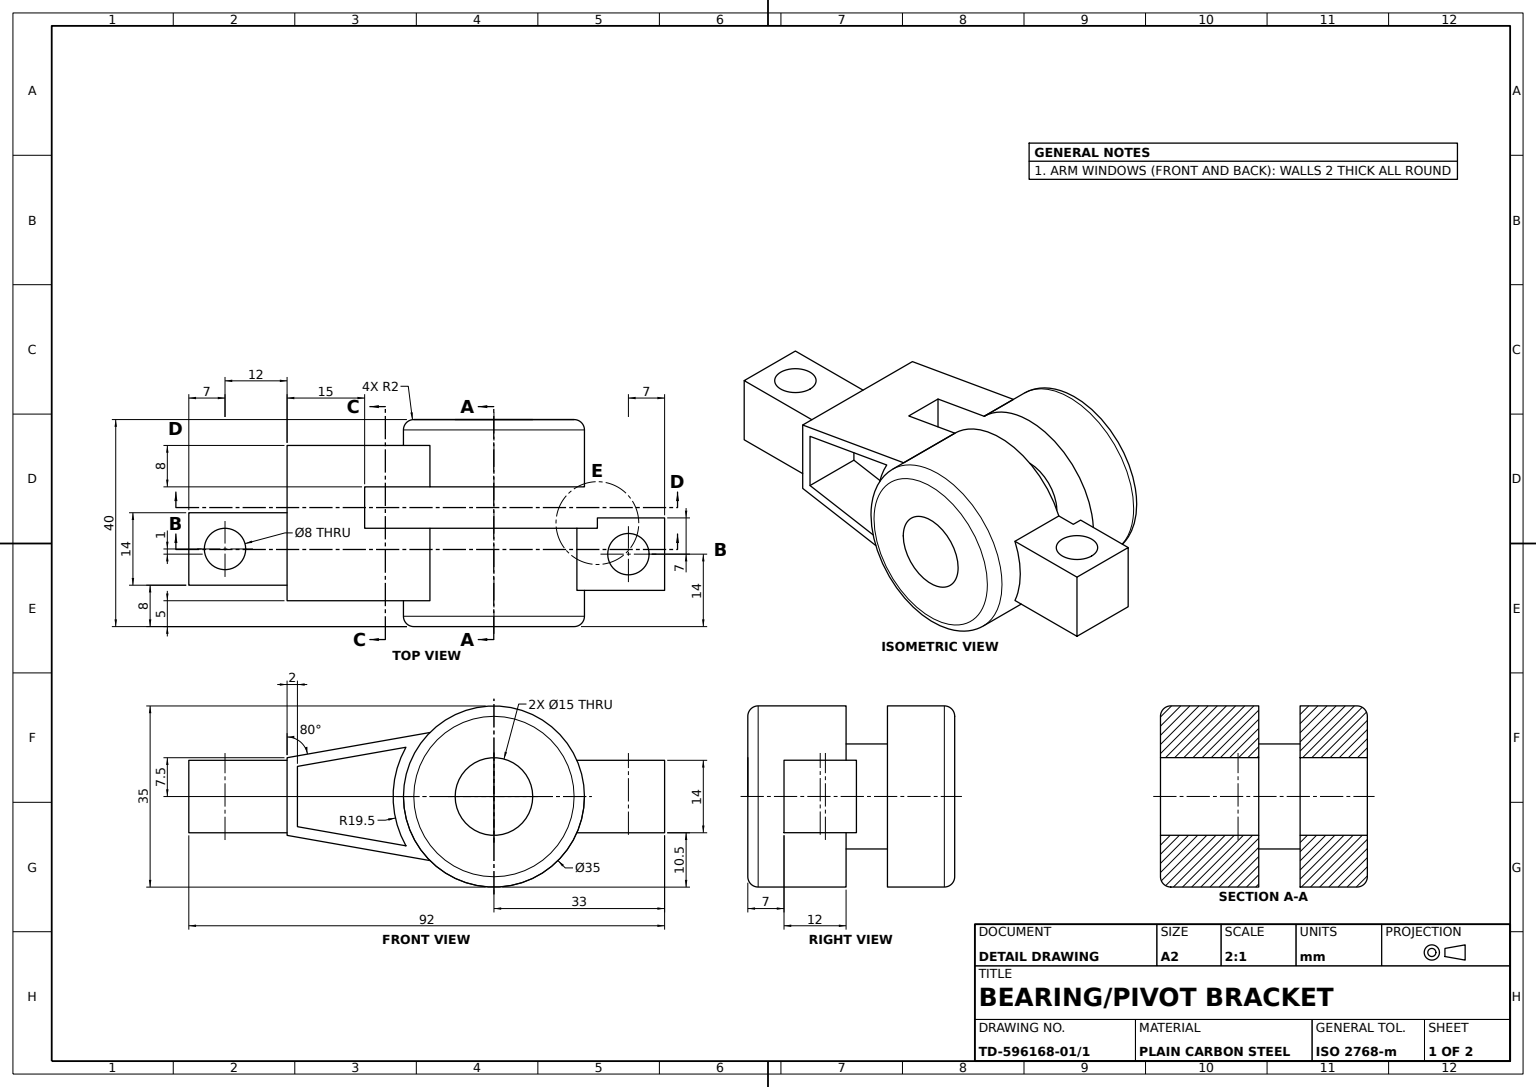
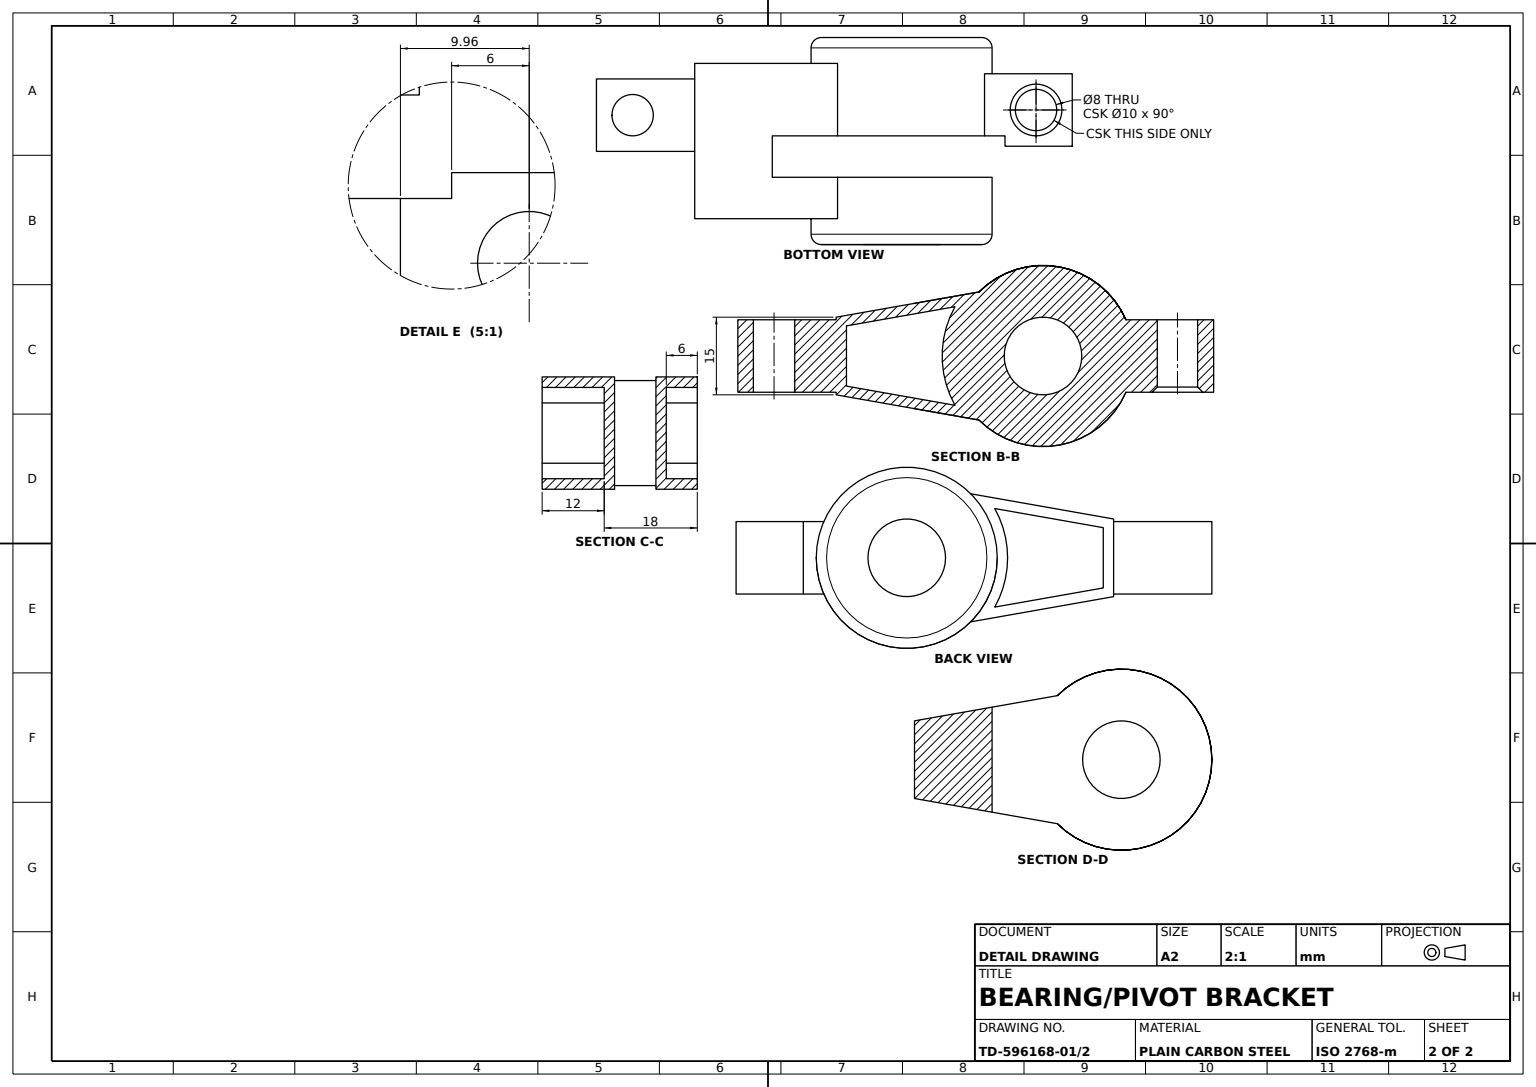
SolidWorks part; units mm, degrees
material "Plain Carbon Steel"
ref_plane "Front Plane" through (0, 0, 0) normal (0, 0, 1) x (1, 0, 0)
ref_plane "Top Plane" through (0, 0, 0) normal (0, 1, 0) x (1, 0, 0)
ref_plane "Right Plane" through (0, 0, 0) normal (1, 0, 0) x (0, 0, -1)
sketch "Bracket Side Profile Sketch" plane through (0, 0, 0) normal (0, 0, 1) x (1, 0, 0)
  line L0 (-46, 0) -> (46, 0) construction
  line L1 (-46, -7) -> (-46, 7)
  line L2 (-46, 7) -> (-27, 7)
  line L3 (-27, 7) -> (-27, 7.5)
  line L4 (-27, 7.5) -> (0.6217, 12.3705)
  line L5 (-46, -7) -> (-27, -7)
  line L6 (-27, -7.5) -> (0.6217, -12.3705)
  line L7 (46, -7) -> (46, 7)
  line L8 (46, 7) -> (29.039, 7)
  line L9 (46, -7) -> (29.039, -7)
  line L10 (-27, -7) -> (-27, -7.5)
  arc A0 (0.6217, -12.3705) -> (29.039, -7) centre (13, 0) ccw
  circle A1 centre (13, 0) radius 7.5
  arc A2 (29.039, 7) -> (0.6217, 12.3705) centre (13, 0) ccw
  point P3 (0, 0)
  dimension "D2" = 35
  dimension "D3" = 15
  dimension "D1" = 92
  dimension "D4" = 19
  dimension "D5" = 7
  dimension "D6" = 40
  dimension "D7" = 7.5
  dimension "D8" = 80
  dimension "D9" = 7
extrude "Bracket Body 40mm" add sketch "Bracket Side Profile Sketch" along normal mid plane 40
sketch "Top Slot Sketch" plane through (0, 0, 0) normal (0, 1, 0) x (1, 0, 0)
  line L0 (-27, -20) -> (-27, 20) construction
  line L1 (-12, 7) -> (33, 7)
  line L2 (-12, 7) -> (-12, -1)
  line L3 (-12, -1) -> (33, -1)
  line L4 (33, 7) -> (33, -1)
  line L5 (0.6217, -20) -> (29.039, -20) construction
  line L6 (46, -20) -> (46, 20) construction
  dimension "D1" = 15
  dimension "D2" = 19
  dimension "D3" = 8
  dimension "D4" = 13
extrude "Top Slot Cut 15x19" cut sketch "Top Slot Sketch" against normal through all both and the other way through all
sketch "Side Relief A Sketch" plane through (0, 0, 20) normal (0, 0, 1) x (1, 0, 0)
  line L0 (29.039, -7) -> (46, -7) construction
  line L1 (46, -7) -> (46, 7) construction
  line L2 (46, 7) -> (29.039, 7) construction
  line L3 (29.039, -7) -> (46, -7)
  line L4 (46, -7) -> (46, 7)
  line L5 (46, 7) -> (29.039, 7)
  arc A0 (29.039, -7) -> (29.039, 7) centre (13, 0) ccw
extrude "Side Relief A Cut 7mm" cut sketch "Side Relief A Sketch" against normal blind 7
sketch "Side Relief B Sketch" plane through (0, 0, 20) normal (0, 0, 1) x (1, 0, 0)
  line L0 (-27, 7) -> (-27, -7)
  line L1 (-27, -7) -> (-46, -7)
  line L2 (-46, -7) -> (-46, 7)
  line L3 (-46, 7) -> (-27, 7)
extrude "Side Relief B Cut 7mm" cut sketch "Side Relief B Sketch" against normal blind 7
sketch "Lug Trim A Sketch" plane through (0, 0, 20) normal (0, 0, 1) x (1, 0, 0)
  line L0 (-27, -7) -> (-27, 7) construction
  line L1 (-27, -7) -> (-27, 7)
  line L3 (-27, 7.5) -> (-27, -7.5)
  line L4 (-27, -7.5) -> (0.6217, -12.3705)
  line L5 (0.6217, 12.3705) -> (-27, 7.5)
  line L6 (-27, 7.5) -> (-27, -7.5)
  line L7 (-27, -7.5) -> (0.6217, -12.3705)
  line L8 (0.6217, 12.3705) -> (-27, 7.5)
  arc A0 (0.6217, 12.3705) -> (0.6217, -12.3705) centre (13, 0) ccw
  arc A2 (0.6217, -12.3705) -> (0.6217, 12.3705) centre (13, 0) ccw
  line M6 (-27, 7.5) -> (-27, -7.5)
  line M7 (-27, -7.5) -> (0.6217, -12.3705)
  line M9 (0.6217, 12.3705) -> (-27, 7.5)
  dimension "D1" = 0
extrude "Lug Trim A Cut 5mm" cut sketch "Lug Trim A Sketch" against normal blind 5 contours A0 M9 M6 M7
sketch "Lug Trim B Sketch" plane through (0, 0, -20) normal (0, 0, -1) x (-1, 0, 0)
  line L0 (-0.6217, 12.3705) -> (27, 7.5) construction
  line L1 (27, -7.5) -> (-0.6217, -12.3705) construction
  line L2 (27, -7.5) -> (-0.6217, -12.3705)
  line L3 (-0.6217, 12.3705) -> (27, 7.5)
  line L4 (27, 7.5) -> (27, -7.5)
  arc A0 (-0.6217, -12.3705) -> (-0.6217, 12.3705) centre (-13, 0) ccw
extrude "Lug Trim B Cut 5mm" cut sketch "Lug Trim B Sketch" against normal blind 5
sketch "Hub Gap Sketch" plane through (0, 0, -20) normal (0, 0, -1) x (-1, 0, 0)
  line L4 (46, 7) -> (27, 7)
  line L5 (27, 7) -> (27, -7)
  line L6 (27, -7) -> (46, -7)
  line L7 (46, -7) -> (46, 7)
  line L8 (46, 7) -> (27, 7)
  line L9 (27, 7) -> (27, -7)
  line L10 (27, -7) -> (46, -7)
  line L11 (46, -7) -> (46, 7)
  dimension "D1" = 0
extrude "Hub Gap Cut 18mm" cut sketch "Hub Gap Sketch" against normal blind 18
sketch "Relief Step Sketch" plane through (0, 0, 13) normal (0, 0, 1) x (1, 0, 0)
  line L4 (-27, 7) -> (-46, 7)
  line L5 (-46, 7) -> (-46, -7)
  line L6 (-46, -7) -> (-27, -7)
  line L7 (-27, -7) -> (-27, 7)
  line L8 (-27, 7) -> (-46, 7)
  line L9 (-46, 7) -> (-46, -7)
  line L10 (-46, -7) -> (-27, -7)
  line L11 (-27, -7) -> (-27, 7)
  dimension "D1" = 0
extrude "Relief Step Cut 1mm" cut sketch "Relief Step Sketch" against normal blind 1
sketch "Window Opening Sketch" plane through (0, 0, -20) normal (0, 0, -1) x (-1, 0, 0)
  line L0 (-29.039, 7) -> (-46, 7)
  line L1 (-46, 7) -> (-46, -7)
  line L2 (-46, -7) -> (-29.039, -7)
  arc A0 (-29.039, 7) -> (-29.039, -7) centre (-13, 0) ccw
extrude "Window Opening Cut 19mm" cut sketch "Window Opening Sketch" against normal blind 19
sketch "Lug Hole A Sketch" plane through (0, 0, 15) normal (0, 0, 1) x (1, 0, 0)
  line L15 (-4.0173, 9.5216) -> (-25, 5.8218)
  line L16 (-25, 5.8218) -> (-25, -5.8218)
  line L17 (-25, -5.8218) -> (-4.0173, -9.5216)
  line L18 (-4.0173, 9.5216) -> (-25, 5.8218)
  line L19 (-25, 5.8218) -> (-25, -5.8218)
  line L20 (-25, -5.8218) -> (-4.0173, -9.5216)
  arc A5 (-4.0173, 9.5216) -> (-4.0173, -9.5216) centre (13, 0) ccw
  arc A6 (-4.0173, 9.5216) -> (-4.0173, -9.5216) centre (13, 0) ccw
  dimension "D1" = 2
extrude "Lug Hole A Cut 12mm" cut sketch "Lug Hole A Sketch" against normal blind 12
sketch "Lug Hole B Sketch" plane through (0, 0, -15) normal (0, 0, -1) x (-1, 0, 0)
  line L6 (4.0173, -9.5216) -> (25, -5.8218)
  line L7 (25, -5.8218) -> (25, 5.8218)
  line L8 (25, 5.8218) -> (4.0173, 9.5216)
  line L9 (4.0173, -9.5216) -> (25, -5.8218)
  line L10 (25, -5.8218) -> (25, 5.8218)
  line L11 (25, 5.8218) -> (4.0173, 9.5216)
  arc A2 (4.0173, -9.5216) -> (4.0173, 9.5216) centre (-13, 0) ccw
  arc A3 (4.0173, -9.5216) -> (4.0173, 9.5216) centre (-13, 0) ccw
  dimension "D1" = 2
extrude "Lug Hole B Cut 6mm" cut sketch "Lug Hole B Sketch" against normal blind 6
fillet "Edge Fillet R2" radius 2 2 edges at (30.5, 0, 20) (30.5, 0, -20)
sketch "Hub Bore Sketch" plane through (0, 7, 0) normal (0, 1, 0) x (1, 0, 0)
  line L1 (33, 1) -> (46, 1) construction
  line L2 (46, -13) -> (46, 1) construction
  line L3 (-46, -12) -> (-46, 2) construction
  line L4 (-46, 2) -> (-27, 2) construction
  circle A0 centre (-39, -5) radius 4
  circle A1 centre (39, -6) radius 4
  dimension "D1" = 7
  dimension "D5" = 8
  dimension "D2" = 7
  dimension "D3" = 7
  dimension "D4" = 7
extrude "Hub Bore Cut" cut sketch "Hub Bore Sketch" against normal up to next
chamfer "Bore Chamfer 1x45" distance 1 angle 45 1 edges at (35, -7, 6)
